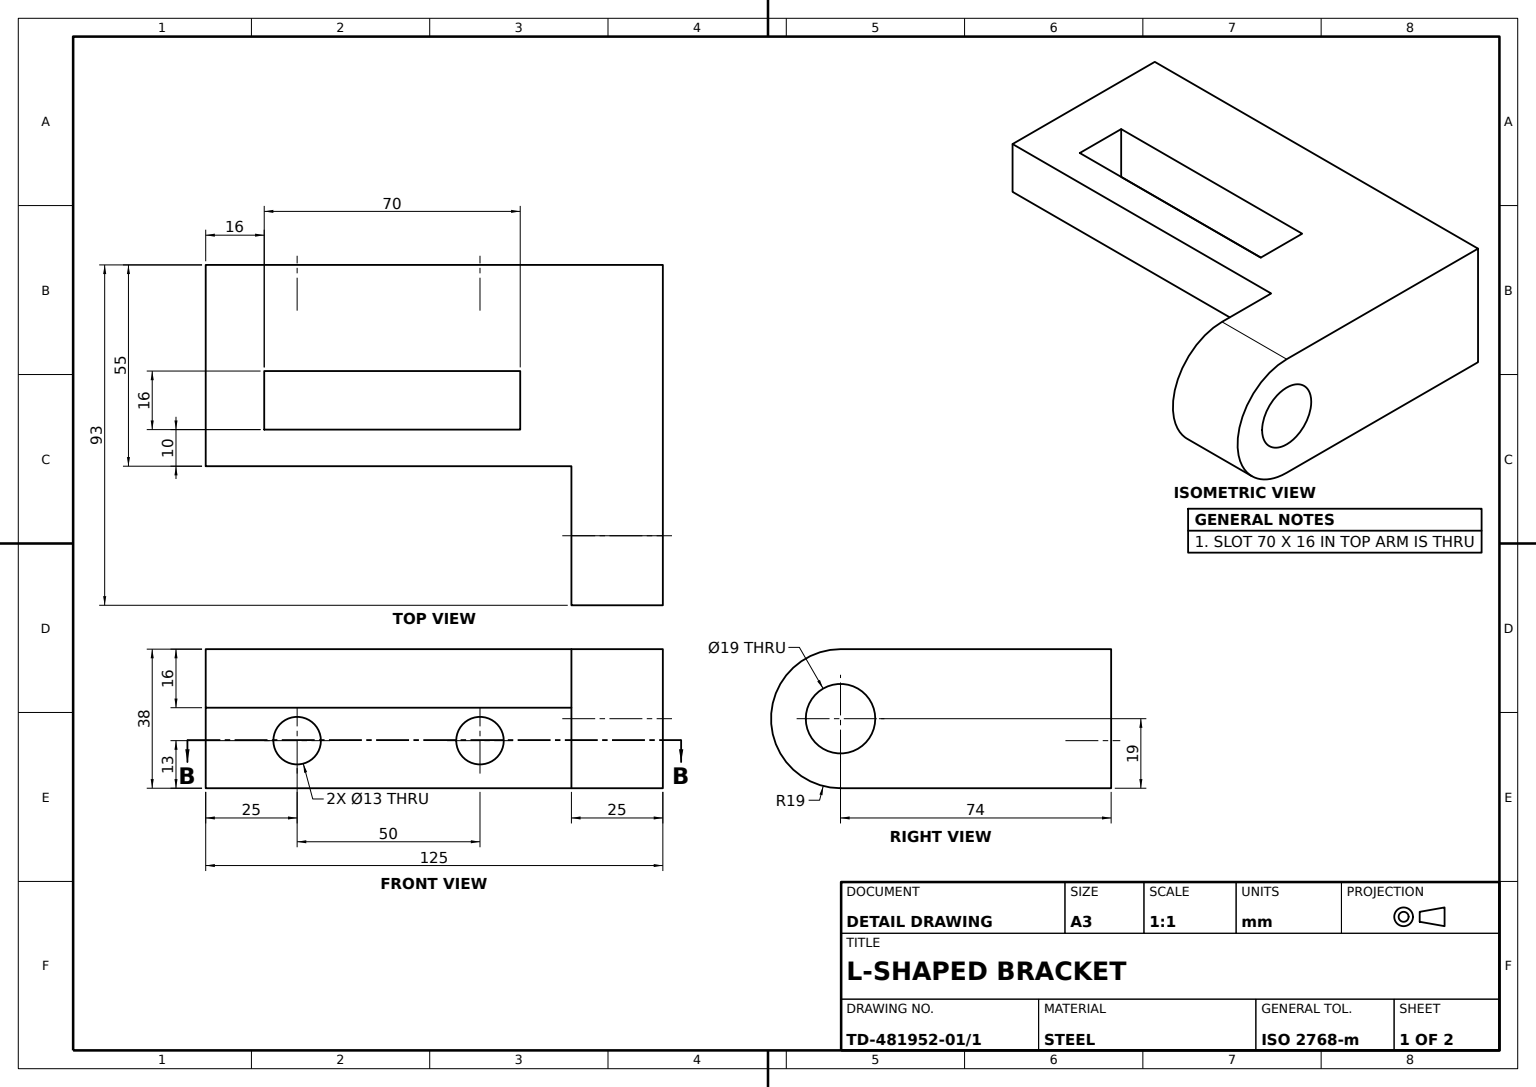
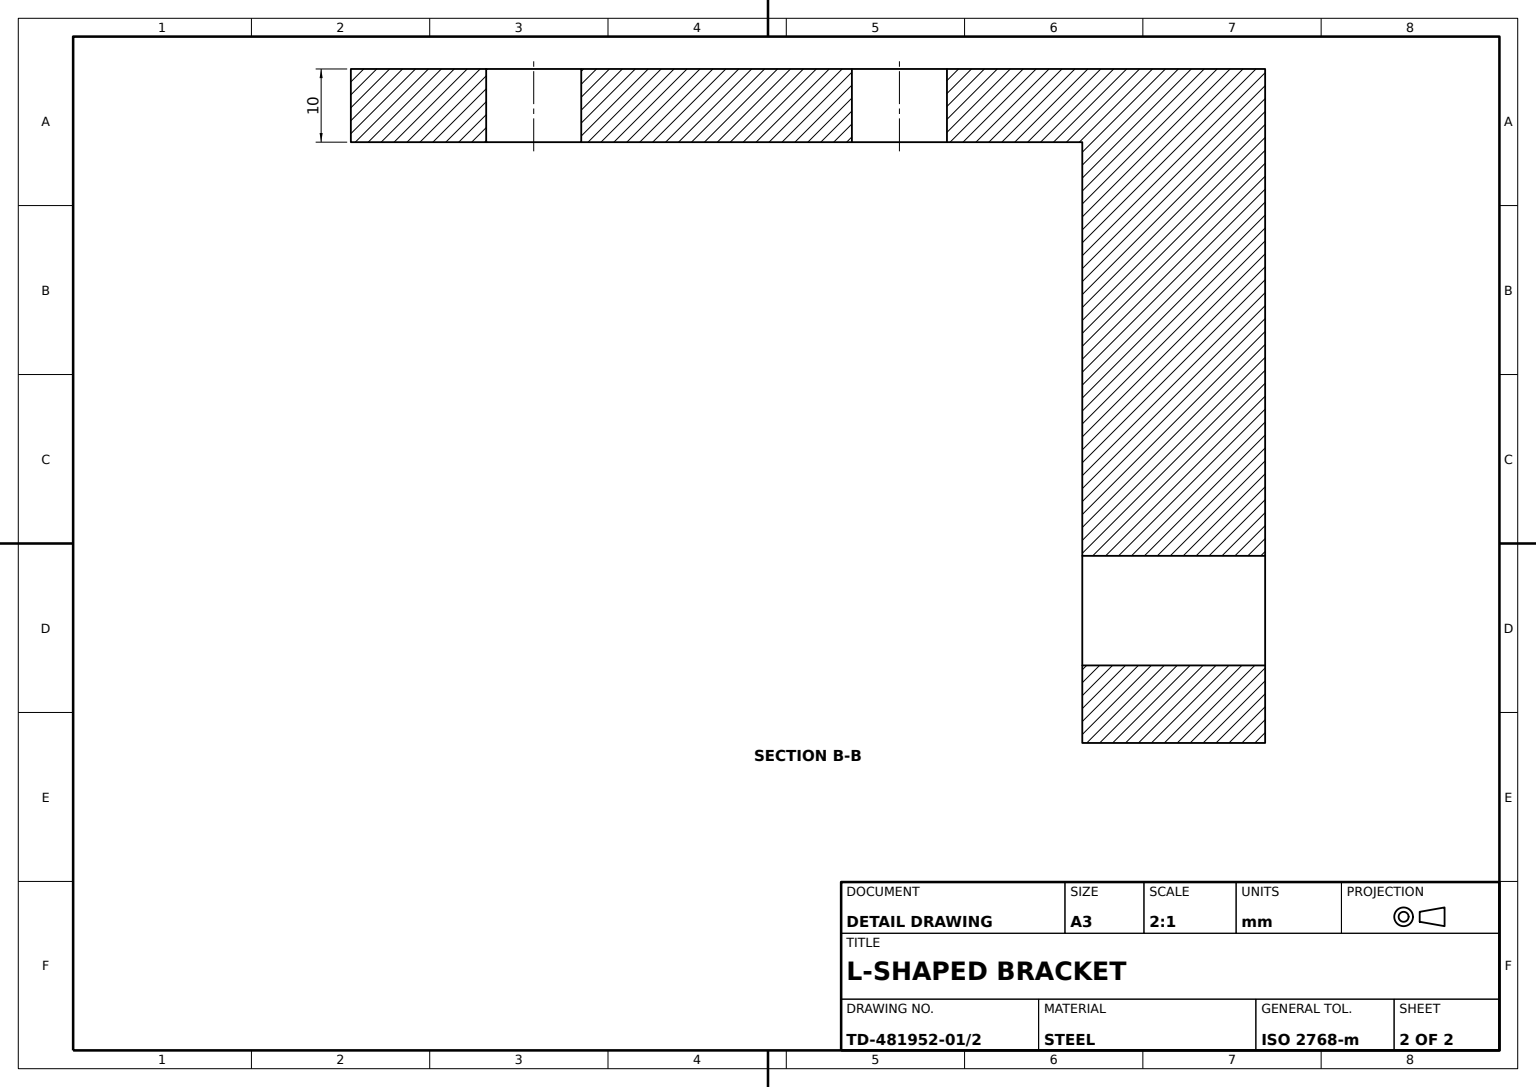
SolidWorks part; units mm, degrees
material "Plain Carbon Steel"
ref_plane "Front Plane" through (0, 0, 0) normal (0, 0, 1) x (1, 0, 0)
ref_plane "Top Plane" through (0, 0, 0) normal (0, 1, 0) x (1, 0, 0)
ref_plane "Right Plane" through (0, 0, 0) normal (1, 0, 0) x (0, 0, -1)
sketch "Base Plate Sketch" plane through (0, 0, 0) normal (0, 0, 1) x (1, 0, 0)
  line L0 (0, 0) -> (125, 0)
  line L1 (125, 0) -> (125, 38)
  line L2 (125, 38) -> (0, 38)
  line L3 (0, 38) -> (0, 0)
  dimension "D1" = 125
  dimension "D2" = 38
extrude "Base Plate" add sketch "Base Plate Sketch" along normal blind 10
sketch "Hinge Lug Sketch" plane through (125, 0, 0) normal (1, 0, 0) x (0, 0, -1)
  line L0 (-10, 38) -> (-74, 38)
  line L2 (-74, 0) -> (-10, 0)
  line L3 (-10, 0) -> (-10, 38)
  line L4 (0, 0) -> (0, 38) construction
  arc A0 (-74, 38) -> (-74, 0) centre (-74, 19) ccw
  dimension "D1" = 38
  dimension "D2" = 74
extrude "Hinge Lug" add sketch "Hinge Lug Sketch" against normal blind 25
sketch "Lug Bore Ø19 Sketch" plane through (125, 0, 0) normal (1, 0, 0) x (0, 0, -1)
  circle A0 centre (-74, 19) radius 9.5
  dimension "D1" = 19
  dimension "D2" = 19
extrude "Lug Bore Ø19" cut sketch "Lug Bore Ø19 Sketch" against normal blind 25
sketch "Arm Sketch" plane through (0, 38, 0) normal (0, 1, 0) x (1, 0, 0)
  line L0 (0, -10) -> (0, -55)
  line L1 (0, -55) -> (100, -55)
  line L2 (100, -10) -> (100, -74) construction
  line L3 (100, -55) -> (100, -10)
  line L4 (100, -10) -> (0, -10) construction
  line L5 (100, -10) -> (0, -10)
  line L7 (125, 0) -> (0, 0) construction
  dimension "D1" = 55
extrude "Arm" add sketch "Arm Sketch" against normal blind 16
sketch "Slot 70x16 Sketch" plane through (0, 38, 0) normal (0, 1, 0) x (1, 0, 0)
  line L0 (0, -55) -> (100, -55) construction
  line L1 (16, -29) -> (86, -29)
  line L2 (16, -29) -> (16, -45)
  line L3 (16, -45) -> (86, -45)
  line L4 (86, -29) -> (86, -45)
  line L5 (0, -55) -> (0, 0) construction
  dimension "D1" = 70
  dimension "D2" = 16
  dimension "D3" = 10
  dimension "D4" = 16
extrude "Slot 70x16" cut sketch "Slot 70x16 Sketch" against normal blind 16
sketch "Corner Notch Sketch" plane through (0, 0, 10) normal (0, 0, 1) x (1, 0, 0)
  line L0 (0, 22) -> (0, 0) construction
  line L1 (0, 0) -> (100, 0) construction
  circle A0 centre (25, 13) radius 6.5
  circle A1 centre (75, 13) radius 6.5
  dimension "D1" = 13
  dimension "D2" = 25
  dimension "D4" = 13
  dimension "D6" = 13
  dimension "D3" = 13
  dimension "D5" = 50
extrude "Corner Notch" cut sketch "Corner Notch Sketch" against normal blind 10
